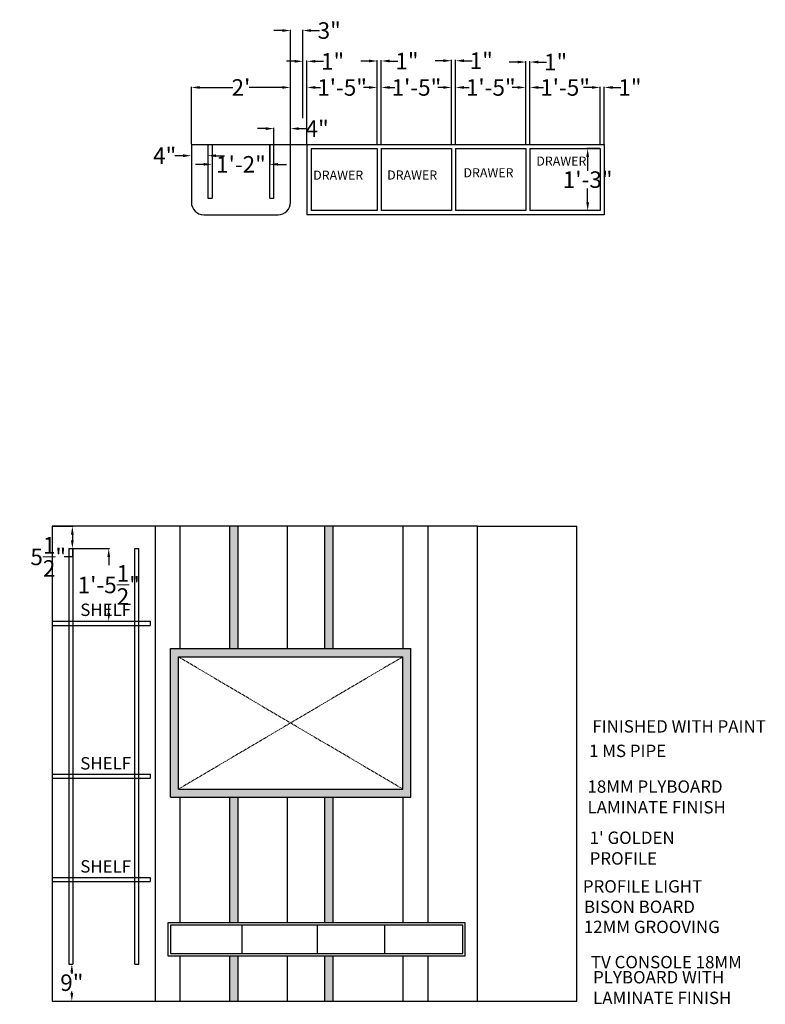
# Model space of a CAD drawing. Units: inches. Extents: x 40 to 220, y 34 to 272.
import ezdxf

# ---------------------------------------------------------------- set-up
doc = ezdxf.new("R2010")
doc.units = ezdxf.units.IN
doc.header["$MEASUREMENT"] = 0
doc.linetypes.add('CENTER2', pattern=[1.125, 0.75, -0.125, 0.125, -0.125])
for name, color, linetype, lineweight in [('A-ANNO-DIMS', 2, 'Continuous', 18), ('A-ANNO-TEXT', 7, 'Continuous', 18), ('A-EQPM', 8, 'CENTER2', 18), ('A-FURN', 7, 'Continuous', 25), ('A-FURN-PATT', 30, 'Continuous', 13)]:
    doc.layers.add(name, color=color, linetype=linetype, lineweight=lineweight)
doc.styles.get("Standard").update_dxf_attribs({"font": 'arial.ttf'})
doc.dimstyles.get("Standard").update_dxf_attribs({"dimtxt": 4, "dimasz": 2, "dimexe": 0.18, "dimexo": 0.0625, "dimgap": 0.09, "dimtad": 0, "dimtih": 1, "dimtoh": 1, "dimdec": 1, "dimzin": 0, "dimdsep": 46, "dimlunit": 4, "dimtxsty": 'Standard', "dimcen": 0.09, "dimadec": 0, "dimazin": 0, "dimtfac": 1, "dimtdec": 1, "dimtofl": 0, "dimtmove": 0, "dimatfit": 3, "dimfxl": 1, "dimtolj": 1, "dimtzin": 0, "dimarcsym": 1})

# ---------------------------------------------------------------- blocks, each defined once
blk = doc.blocks.new('*D1')
at = {"layer": 'A-ANNO-DIMS', "color": 0, "lineweight": -2, "transparency": 16777216}
for p, q in [((81.22, 241.93), (81.22, 255.87)), ((83.22, 255.69), (91.25, 255.69)), ((103.22, 255.69), (95.18, 255.69)), ((105.22, 241.93), (105.22, 255.87))]:
    blk.add_line(p, q, dxfattribs=at)
at = {"layer": 'A-ANNO-DIMS', "color": 0, "transparency": 16777216}
for points in [[(83.22, 256.02), (83.22, 255.36), (81.22, 255.69)], [(103.22, 256.02), (103.22, 255.36), (105.22, 255.69)]]:
    blk.add_solid(points, dxfattribs=at)
at = {"layer": 'Defpoints', "color": 0, "transparency": 16777216}
for p in [(105.22, 255.69), (81.22, 241.87), (105.22, 241.87)]:
    blk.add_point(p, dxfattribs=at)
at = {"layer": 'A-ANNO-DIMS', "color": 0, "transparency": 16777216, "insert": (93.22, 255.69), "char_height": 4, "attachment_point": 5}
blk.add_mtext("\\A1;2'", dxfattribs=at)
blk = doc.blocks.new('*D2')
at = {"layer": 'A-ANNO-DIMS', "color": 0, "lineweight": -2, "transparency": 16777216}
for p, q in [((103.22, 269.47), (101.22, 269.47)), ((105.22, 255.72), (105.22, 269.65)), ((108.22, 255.72), (108.22, 269.65)), ((110.22, 269.47), (112.22, 269.47))]:
    blk.add_line(p, q, dxfattribs=at)
at = {"layer": 'A-ANNO-DIMS', "color": 0, "transparency": 16777216}
for points in [[(103.22, 269.8), (103.22, 269.14), (105.22, 269.47)], [(110.22, 269.8), (110.22, 269.14), (108.22, 269.47)]]:
    blk.add_solid(points, dxfattribs=at)
at = {"layer": 'Defpoints', "color": 0, "transparency": 16777216}
for p in [(108.22, 269.47), (105.22, 255.65), (108.22, 255.65)]:
    blk.add_point(p, dxfattribs=at)
at = {"layer": 'A-ANNO-DIMS', "color": 0, "transparency": 16777216, "insert": (114.6, 269.47), "char_height": 4, "attachment_point": 5}
blk.add_mtext('\\A1;3"', dxfattribs=at)
blk = doc.blocks.new('*D3')
at = {"layer": 'A-ANNO-DIMS', "color": 0, "lineweight": -2, "transparency": 16777216}
for p, q in [((106.22, 262.02), (104.22, 262.02)), ((108.22, 248.27), (108.22, 262.2)), ((109.22, 248.27), (109.22, 262.2)), ((111.22, 262.02), (113.22, 262.02))]:
    blk.add_line(p, q, dxfattribs=at)
at = {"layer": 'A-ANNO-DIMS', "color": 0, "transparency": 16777216}
for points in [[(106.22, 262.35), (106.22, 261.69), (108.22, 262.02)], [(111.22, 262.35), (111.22, 261.69), (109.22, 262.02)]]:
    blk.add_solid(points, dxfattribs=at)
at = {"layer": 'Defpoints', "color": 0, "transparency": 16777216}
for p in [(109.22, 262.02), (108.22, 248.2), (109.22, 248.2)]:
    blk.add_point(p, dxfattribs=at)
at = {"layer": 'A-ANNO-DIMS', "color": 0, "transparency": 16777216, "insert": (115.42, 262.02), "char_height": 4, "attachment_point": 5}
blk.add_mtext('\\A1;1"', dxfattribs=at)
blk = doc.blocks.new('*D4')
at = {"layer": 'A-ANNO-DIMS', "color": 0, "lineweight": -2, "transparency": 16777216}
for p, q in [((109.22, 241.93), (109.22, 255.87)), ((111.22, 255.69), (112.5, 255.69)), ((124.22, 255.69), (122.93, 255.69)), ((126.22, 241.93), (126.22, 255.87))]:
    blk.add_line(p, q, dxfattribs=at)
at = {"layer": 'A-ANNO-DIMS', "color": 0, "transparency": 16777216}
for points in [[(111.22, 256.02), (111.22, 255.36), (109.22, 255.69)], [(124.22, 256.02), (124.22, 255.36), (126.22, 255.69)]]:
    blk.add_solid(points, dxfattribs=at)
at = {"layer": 'Defpoints', "color": 0, "transparency": 16777216}
for p in [(126.22, 255.69), (109.22, 241.87), (126.22, 241.87)]:
    blk.add_point(p, dxfattribs=at)
at = {"layer": 'A-ANNO-DIMS', "color": 0, "transparency": 16777216, "insert": (117.72, 255.69), "char_height": 4, "attachment_point": 5}
blk.add_mtext('\\A1;1\'-5"', dxfattribs=at)
blk = doc.blocks.new('*D5')
at = {"layer": 'A-ANNO-DIMS', "color": 0, "lineweight": -2, "transparency": 16777216}
for p, q in [((126.22, 248.34), (126.22, 262.27)), ((127.22, 248.34), (127.22, 262.27)), ((124.22, 262.09), (122.22, 262.09)), ((129.22, 262.09), (131.22, 262.09))]:
    blk.add_line(p, q, dxfattribs=at)
at = {"layer": 'A-ANNO-DIMS', "color": 0, "transparency": 16777216}
for points in [[(124.22, 262.43), (124.22, 261.76), (126.22, 262.09)], [(129.22, 262.43), (129.22, 261.76), (127.22, 262.09)]]:
    blk.add_solid(points, dxfattribs=at)
at = {"layer": 'Defpoints', "color": 0, "transparency": 16777216}
for p in [(127.22, 262.09), (126.22, 248.28), (127.22, 248.28)]:
    blk.add_point(p, dxfattribs=at)
at = {"layer": 'A-ANNO-DIMS', "color": 0, "transparency": 16777216, "insert": (133.42, 262.09), "char_height": 4, "attachment_point": 5}
blk.add_mtext('\\A1;1"', dxfattribs=at)
blk = doc.blocks.new('*D6')
at = {"layer": 'A-ANNO-DIMS', "color": 0, "lineweight": -2, "transparency": 16777216}
for p, q in [((127.22, 241.93), (127.22, 255.87)), ((129.22, 255.69), (130.5, 255.69)), ((142.22, 255.69), (140.93, 255.69)), ((144.22, 241.93), (144.22, 255.87))]:
    blk.add_line(p, q, dxfattribs=at)
at = {"layer": 'A-ANNO-DIMS', "color": 0, "transparency": 16777216}
for points in [[(129.22, 256.02), (129.22, 255.36), (127.22, 255.69)], [(142.22, 256.02), (142.22, 255.36), (144.22, 255.69)]]:
    blk.add_solid(points, dxfattribs=at)
at = {"layer": 'Defpoints', "color": 0, "transparency": 16777216}
for p in [(144.22, 255.69), (127.22, 241.87), (144.22, 241.87)]:
    blk.add_point(p, dxfattribs=at)
at = {"layer": 'A-ANNO-DIMS', "color": 0, "transparency": 16777216, "insert": (135.72, 255.69), "char_height": 4, "attachment_point": 5}
blk.add_mtext('\\A1;1\'-5"', dxfattribs=at)
blk = doc.blocks.new('*D7')
at = {"layer": 'A-ANNO-DIMS', "color": 0, "lineweight": -2, "transparency": 16777216}
for p, q in [((144.22, 248.41), (144.22, 262.34)), ((145.22, 248.41), (145.22, 262.34)), ((142.22, 262.16), (140.22, 262.16)), ((147.22, 262.16), (149.22, 262.16))]:
    blk.add_line(p, q, dxfattribs=at)
at = {"layer": 'A-ANNO-DIMS', "color": 0, "transparency": 16777216}
for points in [[(142.22, 262.5), (142.22, 261.83), (144.22, 262.16)], [(147.22, 262.5), (147.22, 261.83), (145.22, 262.16)]]:
    blk.add_solid(points, dxfattribs=at)
at = {"layer": 'Defpoints', "color": 0, "transparency": 16777216}
for p in [(145.22, 262.16), (144.22, 248.35), (145.22, 248.35)]:
    blk.add_point(p, dxfattribs=at)
at = {"layer": 'A-ANNO-DIMS', "color": 0, "transparency": 16777216, "insert": (151.42, 262.16), "char_height": 4, "attachment_point": 5}
blk.add_mtext('\\A1;1"', dxfattribs=at)
blk = doc.blocks.new('*D8')
at = {"layer": 'A-ANNO-DIMS', "color": 0, "lineweight": -2, "transparency": 16777216}
for p, q in [((145.22, 241.93), (145.22, 255.87)), ((147.22, 255.69), (148.5, 255.69)), ((160.22, 255.69), (158.93, 255.69)), ((162.22, 241.93), (162.22, 255.87))]:
    blk.add_line(p, q, dxfattribs=at)
at = {"layer": 'A-ANNO-DIMS', "color": 0, "transparency": 16777216}
for points in [[(147.22, 256.02), (147.22, 255.36), (145.22, 255.69)], [(160.22, 256.02), (160.22, 255.36), (162.22, 255.69)]]:
    blk.add_solid(points, dxfattribs=at)
at = {"layer": 'Defpoints', "color": 0, "transparency": 16777216}
for p in [(162.22, 255.69), (145.22, 241.87), (162.22, 241.87)]:
    blk.add_point(p, dxfattribs=at)
at = {"layer": 'A-ANNO-DIMS', "color": 0, "transparency": 16777216, "insert": (153.72, 255.69), "char_height": 4, "attachment_point": 5}
blk.add_mtext('\\A1;1\'-5"', dxfattribs=at)
blk = doc.blocks.new('*D9')
at = {"layer": 'A-ANNO-DIMS', "color": 0, "lineweight": -2, "transparency": 16777216}
for p, q in [((160.22, 261.84), (158.22, 261.84)), ((162.22, 248.08), (162.22, 262.02)), ((163.22, 248.08), (163.22, 262.02)), ((165.22, 261.84), (167.22, 261.84))]:
    blk.add_line(p, q, dxfattribs=at)
at = {"layer": 'A-ANNO-DIMS', "color": 0, "transparency": 16777216}
for points in [[(160.22, 262.17), (160.22, 261.51), (162.22, 261.84)], [(165.22, 262.17), (165.22, 261.51), (163.22, 261.84)]]:
    blk.add_solid(points, dxfattribs=at)
at = {"layer": 'Defpoints', "color": 0, "transparency": 16777216}
for p in [(163.22, 261.84), (162.22, 248.02), (163.22, 248.02)]:
    blk.add_point(p, dxfattribs=at)
at = {"layer": 'A-ANNO-DIMS', "color": 0, "transparency": 16777216, "insert": (169.42, 261.84), "char_height": 4, "attachment_point": 5}
blk.add_mtext('\\A1;1"', dxfattribs=at)
blk = doc.blocks.new('*D10')
at = {"layer": 'A-ANNO-DIMS', "color": 0, "lineweight": -2, "transparency": 16777216}
for p, q in [((163.22, 241.93), (163.22, 255.87)), ((165.22, 255.69), (166.5, 255.69)), ((178.22, 255.69), (176.93, 255.69)), ((180.22, 241.93), (180.22, 255.87))]:
    blk.add_line(p, q, dxfattribs=at)
at = {"layer": 'A-ANNO-DIMS', "color": 0, "transparency": 16777216}
for points in [[(165.22, 256.02), (165.22, 255.36), (163.22, 255.69)], [(178.22, 256.02), (178.22, 255.36), (180.22, 255.69)]]:
    blk.add_solid(points, dxfattribs=at)
at = {"layer": 'Defpoints', "color": 0, "transparency": 16777216}
for p in [(180.22, 255.69), (163.22, 241.87), (180.22, 241.87)]:
    blk.add_point(p, dxfattribs=at)
at = {"layer": 'A-ANNO-DIMS', "color": 0, "transparency": 16777216, "insert": (171.72, 255.69), "char_height": 4, "attachment_point": 5}
blk.add_mtext('\\A1;1\'-5"', dxfattribs=at)
blk = doc.blocks.new('*D11')
at = {"layer": 'A-ANNO-DIMS', "color": 0, "lineweight": -2, "transparency": 16777216}
for p, q in [((178.22, 255.69), (176.22, 255.69)), ((180.22, 241.93), (180.22, 255.87)), ((181.22, 241.93), (181.22, 255.87)), ((183.22, 255.69), (185.22, 255.69))]:
    blk.add_line(p, q, dxfattribs=at)
at = {"layer": 'A-ANNO-DIMS', "color": 0, "transparency": 16777216}
for points in [[(178.22, 256.02), (178.22, 255.36), (180.22, 255.69)], [(183.22, 256.02), (183.22, 255.36), (181.22, 255.69)]]:
    blk.add_solid(points, dxfattribs=at)
at = {"layer": 'Defpoints', "color": 0, "transparency": 16777216}
for p in [(181.22, 255.69), (180.22, 241.87), (181.22, 241.87)]:
    blk.add_point(p, dxfattribs=at)
at = {"layer": 'A-ANNO-DIMS', "color": 0, "transparency": 16777216, "insert": (187.42, 255.69), "char_height": 4, "attachment_point": 5}
blk.add_mtext('\\A1;1"', dxfattribs=at)
blk = doc.blocks.new('*D12')
at = {"layer": 'A-ANNO-DIMS', "color": 0, "lineweight": -2, "transparency": 16777216}
for p, q in [((99.22, 245.72), (97.22, 245.72)), ((101.22, 241.93), (101.22, 245.9)), ((105.22, 241.93), (105.22, 245.9)), ((107.22, 245.72), (109.22, 245.72))]:
    blk.add_line(p, q, dxfattribs=at)
at = {"layer": 'A-ANNO-DIMS', "color": 0, "transparency": 16777216}
for points in [[(99.22, 246.05), (99.22, 245.38), (101.22, 245.72)], [(107.22, 246.05), (107.22, 245.38), (105.22, 245.72)]]:
    blk.add_solid(points, dxfattribs=at)
at = {"layer": 'Defpoints', "color": 0, "transparency": 16777216}
for p in [(105.22, 245.72), (101.22, 241.87), (105.22, 241.87)]:
    blk.add_point(p, dxfattribs=at)
at = {"layer": 'A-ANNO-DIMS', "color": 0, "transparency": 16777216, "insert": (111.68, 245.72), "char_height": 4, "attachment_point": 5}
blk.add_mtext('\\A1;4"', dxfattribs=at)
blk = doc.blocks.new('*D13')
at = {"layer": 'A-ANNO-DIMS', "color": 0, "lineweight": -2, "transparency": 16777216}
for p, q in [((81.22, 241.81), (81.22, 238.98)), ((85.22, 241.81), (85.22, 238.98)), ((79.22, 239.16), (77.22, 239.16)), ((87.22, 239.16), (89.22, 239.16))]:
    blk.add_line(p, q, dxfattribs=at)
at = {"layer": 'A-ANNO-DIMS', "color": 0, "transparency": 16777216}
for points in [[(79.22, 239.5), (79.22, 238.83), (81.22, 239.16)], [(87.22, 239.5), (87.22, 238.83), (85.22, 239.16)]]:
    blk.add_solid(points, dxfattribs=at)
at = {"layer": 'Defpoints', "color": 0, "transparency": 16777216}
for p in [(81.22, 241.87), (85.22, 241.87), (81.22, 239.16)]:
    blk.add_point(p, dxfattribs=at)
at = {"layer": 'A-ANNO-DIMS', "color": 0, "transparency": 16777216, "insert": (74.75, 239.16), "char_height": 4, "attachment_point": 5}
blk.add_mtext('\\A1;4"', dxfattribs=at)
blk = doc.blocks.new('*D14')
at = {"layer": 'A-ANNO-DIMS', "color": 0, "lineweight": -2, "transparency": 16777216}
for p, q in [((86.22, 241.81), (86.22, 236.89)), ((100.22, 241.81), (100.22, 236.89)), ((84.22, 237.07), (82.22, 237.07)), ((102.22, 237.07), (104.22, 237.07))]:
    blk.add_line(p, q, dxfattribs=at)
at = {"layer": 'A-ANNO-DIMS', "color": 0, "transparency": 16777216}
for points in [[(84.22, 237.41), (84.22, 236.74), (86.22, 237.07)], [(102.22, 237.41), (102.22, 236.74), (100.22, 237.07)]]:
    blk.add_solid(points, dxfattribs=at)
at = {"layer": 'Defpoints', "color": 0, "transparency": 16777216}
for p in [(86.22, 241.87), (100.22, 241.87), (100.22, 237.07)]:
    blk.add_point(p, dxfattribs=at)
at = {"layer": 'A-ANNO-DIMS', "color": 0, "transparency": 16777216, "insert": (93.22, 237.07), "char_height": 4, "attachment_point": 5}
blk.add_mtext('\\A1;1\'-2"', dxfattribs=at)
blk = doc.blocks.new('*D15')
at = {"layer": 'A-ANNO-DIMS', "color": 0, "lineweight": -2, "transparency": 16777216}
for p, q in [((180.15, 240.87), (177.01, 240.87)), ((177.19, 238.87), (177.19, 235.51)), ((177.19, 227.87), (177.19, 231.24)), ((180.15, 225.87), (177.01, 225.87))]:
    blk.add_line(p, q, dxfattribs=at)
at = {"layer": 'A-ANNO-DIMS', "color": 0, "transparency": 16777216}
for points in [[(176.85, 238.87), (177.52, 238.87), (177.19, 240.87)], [(176.85, 227.87), (177.52, 227.87), (177.19, 225.87)]]:
    blk.add_solid(points, dxfattribs=at)
at = {"layer": 'Defpoints', "color": 0, "transparency": 16777216}
for p in [(180.22, 240.87), (177.19, 225.87), (180.22, 225.87)]:
    blk.add_point(p, dxfattribs=at)
at = {"layer": 'A-ANNO-DIMS', "color": 0, "transparency": 16777216, "insert": (177.19, 233.37), "char_height": 4, "attachment_point": 5}
blk.add_mtext('\\A1;1\'-3"', dxfattribs=at)
blk = doc.blocks.new('*D16')
at = {"layer": 'A-ANNO-DIMS', "color": 0, "lineweight": -2, "transparency": 16777216}
for p, q in [((47.59, 149.42), (52.58, 149.42)), ((52.4, 147.42), (52.4, 146.02)), ((51.59, 144.02), (52.58, 144.02)), ((52.4, 144.02), (52.4, 142.02)), ((52.4, 142.02), (50.4, 142.02))]:
    blk.add_line(p, q, dxfattribs=at)
at = {"layer": 'A-ANNO-DIMS', "color": 0, "transparency": 16777216}
for points in [[(52.06, 147.42), (52.73, 147.42), (52.4, 149.42)], [(52.06, 146.02), (52.73, 146.02), (52.4, 144.02)]]:
    blk.add_solid(points, dxfattribs=at)
at = {"layer": 'Defpoints', "color": 0, "transparency": 16777216}
for p in [(47.53, 149.42), (51.53, 144.02), (52.4, 144.02)]:
    blk.add_point(p, dxfattribs=at)
at = {"layer": 'A-ANNO-DIMS', "color": 0, "transparency": 16777216, "insert": (46.55, 142.02), "char_height": 4, "attachment_point": 5}
blk.add_mtext('\\A1;5{\\H1x;\\S1/2;}"', dxfattribs=at)
blk = doc.blocks.new('*D17')
at = {"layer": 'A-ANNO-DIMS', "color": 0, "lineweight": -2, "transparency": 16777216}
for p, q in [((52.64, 144.02), (61.39, 144.02)), ((61.21, 142.02), (61.21, 140.02)), ((61.21, 128.42), (61.21, 130.41)), ((52.64, 126.42), (61.39, 126.42))]:
    blk.add_line(p, q, dxfattribs=at)
at = {"layer": 'A-ANNO-DIMS', "color": 0, "transparency": 16777216}
for points in [[(60.88, 142.02), (61.54, 142.02), (61.21, 144.02)], [(60.88, 128.42), (61.54, 128.42), (61.21, 126.42)]]:
    blk.add_solid(points, dxfattribs=at)
at = {"layer": 'Defpoints', "color": 0, "transparency": 16777216}
for p in [(52.58, 144.02), (52.58, 126.42), (61.21, 126.42)]:
    blk.add_point(p, dxfattribs=at)
at = {"layer": 'A-ANNO-DIMS', "color": 0, "transparency": 16777216, "insert": (61.21, 135.22), "char_height": 4, "attachment_point": 5}
blk.add_mtext('\\A1;1\'-5{\\H1x;\\S1/2;}"', dxfattribs=at)
blk = doc.blocks.new('*D18')
at = {"layer": 'A-ANNO-DIMS', "color": 0, "lineweight": -2, "transparency": 16777216}
for p, q in [((51.59, 43.42), (52.45, 43.42)), ((52.27, 41.42), (52.27, 41.05)), ((52.27, 36.42), (52.27, 36.79)), ((47.59, 34.42), (52.45, 34.42))]:
    blk.add_line(p, q, dxfattribs=at)
at = {"layer": 'A-ANNO-DIMS', "color": 0, "transparency": 16777216}
for points in [[(51.94, 41.42), (52.61, 41.42), (52.27, 43.42)], [(51.94, 36.42), (52.61, 36.42), (52.27, 34.42)]]:
    blk.add_solid(points, dxfattribs=at)
at = {"layer": 'Defpoints', "color": 0, "transparency": 16777216}
for p in [(51.53, 43.42), (47.53, 34.42), (52.27, 34.42)]:
    blk.add_point(p, dxfattribs=at)
at = {"layer": 'A-ANNO-DIMS', "color": 0, "transparency": 16777216, "insert": (52.27, 38.92), "char_height": 4, "attachment_point": 5}
blk.add_mtext('\\A1;9"', dxfattribs=at)
blk = doc.blocks.new('DRAWER-FRONT')
for p, q in [((0, 15), (17, 15)), ((0, 15), (0, 0)), ((17, 15), (17, 0)), ((17, 0), (0, 0))]:
    blk.add_line(p, q)
blk = doc.blocks.new('SHELF')
for p, q in [((0, 1), (23.74, 1)), ((0, 0), (23.74, 0)), ((23.74, 1), (23.74, 0))]:
    blk.add_line(p, q)

msp = doc.modelspace()

# ---------------------------------------------------------------- hatches: boundary and pattern name
at = {"layer": 'A-FURN-PATT'}
h = msp.add_hatch(color=256, dxfattribs=at)
h.dxf.hatch_style = 1
h.paths.add_polyline_path([(92.53, 149.42), (90.53, 149.42), (90.53, 119.81), (92.53, 119.81)])
h.paths.add_polyline_path([(115.53, 149.42), (113.53, 149.42), (113.53, 119.81), (115.53, 119.81)])
h.paths.add_polyline_path([(92.53, 83.81), (90.53, 83.81), (90.53, 53.42), (92.53, 53.42)])
h.paths.add_polyline_path([(115.53, 83.81), (113.53, 83.81), (113.53, 53.42), (115.53, 53.42)])
h.paths.add_polyline_path([(115.53, 45.42), (113.53, 45.42), (113.53, 34.42), (115.53, 34.42)])
h.paths.add_polyline_path([(92.53, 45.42), (90.53, 45.42), (90.53, 34.42), (92.53, 34.42)])
h = msp.add_hatch(color=256, dxfattribs=at)
h.dxf.hatch_style = 1
h.paths.add_polyline_path([(134.39, 119.81), (76.13, 119.81), (76.13, 83.81), (134.39, 83.81)])
h.paths.add_polyline_path([(132.39, 117.81), (132.39, 85.81), (78.13, 85.81), (78.13, 117.81)], flags=16)

# ---------------------------------------------------------------- linework, layer by layer
at = {"layer": 'A-EQPM'}
for p, q in [((78.13, 117.81), (132.39, 85.81)), ((132.39, 117.81), (78.13, 85.81))]:
    msp.add_line(p, q, dxfattribs=at)
at = {"layer": 'A-FURN'}
for p, q in [((81.22, 241.87), (105.22, 241.87)), ((81.22, 241.87), (81.22, 227.87)), ((85.22, 241.87), (85.22, 228.87)), ((86.22, 241.87), (86.22, 228.87)), ((100.22, 228.87), (100.22, 241.87)), ((101.22, 228.87), (101.22, 241.87)), ((105.22, 241.87), (108.22, 241.87)), ((105.22, 227.87), (105.22, 241.87)), ((108.22, 241.87), (109.22, 241.87)), ((109.22, 241.87), (126.22, 241.87)), ((109.22, 241.87), (109.22, 224.87)), ((110.22, 240.87), (110.22, 225.87)), ((110.22, 240.87), (126.22, 240.87)), ((126.22, 241.87), (127.22, 241.87)), ((126.22, 240.87), (126.22, 225.87)), ((127.22, 241.87), (144.22, 241.87)), ((144.22, 241.87), (145.22, 241.87)), ((145.22, 241.87), (162.22, 241.87)), ((162.22, 241.87), (163.22, 241.87)), ((163.22, 241.87), (180.22, 241.87)), ((180.22, 241.87), (181.22, 241.87)), ((181.22, 241.87), (181.22, 224.87)), ((85.22, 228.87), (86.22, 228.87)), ((100.22, 228.87), (101.22, 228.87)), ((84.22, 224.87), (102.22, 224.87)), ((181.22, 224.87), (109.22, 224.87)), ((126.22, 225.87), (110.22, 225.87)), ((72.53, 149.42), (47.53, 149.42)), ((47.53, 149.42), (47.53, 34.42)), ((72.53, 34.42), (72.53, 149.42)), ((150.53, 149.42), (72.53, 149.42)), ((78.53, 119.81), (78.53, 149.42)), ((90.53, 119.81), (90.53, 149.42)), ((92.53, 119.81), (92.53, 149.42)), ((104.53, 119.81), (104.53, 149.42)), ((113.53, 119.81), (113.53, 149.42)), ((115.53, 119.81), (115.53, 149.42)), ((132.53, 119.81), (132.53, 149.42)), ((138.53, 53.42), (138.53, 149.42)), ((150.53, 34.42), (150.53, 149.42)), ((150.53, 149.42), (174.53, 149.42)), ((174.53, 34.42), (174.53, 149.42)), ((51.53, 144.02), (52.53, 144.02)), ((51.53, 144.02), (51.53, 43.42)), ((52.53, 144.02), (52.53, 43.42)), ((67.53, 43.42), (67.53, 144.02)), ((67.53, 144.02), (68.53, 144.02)), ((68.53, 43.42), (68.53, 144.02)), ((76.13, 83.81), (76.13, 119.81)), ((76.13, 119.81), (134.39, 119.81)), ((134.39, 83.81), (134.39, 119.81)), ((78.13, 117.81), (132.39, 117.81)), ((78.13, 85.81), (78.13, 117.81)), ((132.39, 85.81), (132.39, 117.81)), ((76.13, 83.81), (134.39, 83.81)), ((78.13, 85.81), (132.39, 85.81)), ((78.53, 53.42), (78.53, 83.81)), ((90.53, 53.42), (90.53, 83.81)), ((92.53, 53.42), (92.53, 83.81)), ((104.53, 53.42), (104.53, 83.81)), ((113.53, 53.42), (113.53, 83.81)), ((115.53, 53.42), (115.53, 83.81)), ((132.53, 53.42), (132.53, 83.81)), ((138.53, 53.42), (138.53, 83.81)), ((93.45, 52.82), (93.45, 46.02)), ((111.7, 52.82), (111.7, 46.02)), ((127.99, 52.82), (127.99, 46.02)), ((78.53, 34.42), (78.53, 45.42)), ((90.53, 34.42), (90.53, 45.42)), ((92.53, 34.42), (92.53, 45.42)), ((104.53, 34.42), (104.53, 45.42)), ((113.53, 34.42), (113.53, 45.42)), ((115.53, 34.42), (115.53, 45.42)), ((132.53, 34.42), (132.53, 45.42)), ((138.53, 34.42), (138.53, 45.42)), ((51.53, 43.42), (52.53, 43.42)), ((67.53, 43.42), (68.53, 43.42)), ((47.53, 34.42), (72.53, 34.42)), ((72.53, 34.42), (78.53, 34.42)), ((78.53, 34.42), (90.53, 34.42)), ((90.53, 34.42), (92.53, 34.42)), ((92.53, 34.42), (104.53, 34.42)), ((104.53, 34.42), (113.53, 34.42)), ((113.53, 34.42), (115.53, 34.42)), ((115.53, 34.42), (132.53, 34.42)), ((132.53, 34.42), (138.53, 34.42)), ((138.53, 34.42), (150.53, 34.42)), ((150.53, 34.42), (174.53, 34.42))]:
    msp.add_line(p, q, dxfattribs=at)
for points in [[(104.53, 53.42), (90.53, 53.42), (78.53, 53.42), (75.53, 53.42), (75.53, 45.42), (78.53, 45.42), (90.53, 45.42), (104.53, 45.42), (115.53, 45.42), (132.53, 45.42), (138.53, 45.42), (147.53, 45.42), (147.53, 53.42), (138.53, 53.42), (132.53, 53.42), (115.53, 53.42), (92.53, 53.42)], [(92.53, 52.82), (90.53, 52.82), (78.53, 52.82), (76.13, 52.82), (76.13, 46.02), (78.53, 46.02), (90.53, 46.02), (104.53, 46.02), (115.53, 46.02), (132.53, 46.02), (138.53, 46.02), (146.93, 46.02), (146.93, 52.82), (138.53, 52.82), (132.53, 52.82), (115.53, 52.82), (76.13, 52.82)]]:
    msp.add_lwpolyline(points, dxfattribs=at)
for centre, start, end in [((84.22, 227.87), 180, 270), ((102.22, 227.87), 270, 0)]:
    msp.add_arc(centre, 3, start, end, dxfattribs=at)

# ---------------------------------------------------------------- block references
for name, p in [('DRAWER-FRONT', (127.22, 225.87)), ('DRAWER-FRONT', (145.22, 225.87)), ('DRAWER-FRONT', (163.22, 225.87)), ('SHELF', (47.53, 125.42)), ('SHELF', (47.53, 88.42)), ('SHELF', (47.53, 63.42))]:
    msp.add_blockref(name, p, dxfattribs=at)

# ---------------------------------------------------------------- texts
at = {"layer": 'A-ANNO-TEXT', "attachment_point": 1}
for s, width, gutter_width, insert, char_height in [('DRAWER', 11.5035, 11, (164.77, 238.96), 2.2), ('DRAWER', 11.5035, 11, (147.12, 236.14), 2.2), ('DRAWER', 11.5035, 11, (110.73, 235.55), 2.2), ('DRAWER', 11.5035, 11, (128.64, 235.59), 2.2), ('SHELF', 12.4336, 15, (54.31, 130.71), 3), ('FINISHED WITH PAINT', 56.6049, 15, (178.33, 102.48), 3), ('1 MS PIPE', 59.8585, 15, (177.53, 96.55), 3), ('SHELF', 12.4336, 15, (54.31, 93.54), 3), ('18MM PLYBOARD\\PLAMINATE FINISH', 49.19, 15, (177.15, 87.9), 3), ("1' GOLDEN \\PPROFILE", 44.5195, 15, (177.67, 75.51), 3), ('SHELF', 12.4336, 15, (54.31, 68.58), 3), ('PROFILE LIGHT', 47.5036, 15, (176.02, 63.74), 3), ('BISON BOARD', 34.9324, 15, (176.3, 58.79), 3), ('12MM GROOVING', 39.0031, 15, (176.26, 53.93), 3), ('TV CONSOLE 18MM', 48.7855, 15, (177.99, 45.4), 3), ('PLYBOARD WITH \\PLAMINATE FINISH', 56.8195, 15, (178.5, 41.74), 3)]:
    msp.add_mtext_dynamic_manual_height_columns(s, width=width, gutter_width=gutter_width, heights=[0], dxfattribs=dict(at, insert=insert, char_height=char_height))

# ---------------------------------------------------------------- dimensions: what is measured, and where the dimension line sits
at = {"layer": 'A-ANNO-DIMS'}
for base, p1, p2, picture, middle in [((108.22, 269.47), (105.22, 255.65), (108.22, 255.65), '*D2', (114.6, 269.47)), ((109.22, 262.02), (108.22, 248.2), (109.22, 248.2), '*D3', (115.42, 262.02)), ((127.22, 262.09), (126.22, 248.28), (127.22, 248.28), '*D5', (133.42, 262.09)), ((145.22, 262.16), (144.22, 248.35), (145.22, 248.35), '*D7', (151.42, 262.16)), ((163.22, 261.84), (162.22, 248.02), (163.22, 248.02), '*D9', (169.42, 261.84)), ((105.22, 255.69), (81.22, 241.87), (105.22, 241.87), '*D1', (93.22, 255.69)), ((126.22, 255.69), (109.22, 241.87), (126.22, 241.87), '*D4', (117.72, 255.69)), ((144.22, 255.69), (127.22, 241.87), (144.22, 241.87), '*D6', (135.72, 255.69)), ((162.22, 255.69), (145.22, 241.87), (162.22, 241.87), '*D8', (153.72, 255.69)), ((180.22, 255.69), (163.22, 241.87), (180.22, 241.87), '*D10', (171.72, 255.69)), ((181.22, 255.69), (180.22, 241.87), (181.22, 241.87), '*D11', (187.42, 255.69)), ((105.22, 245.72), (101.22, 241.87), (105.22, 241.87), '*D12', (111.68, 245.72)), ((81.22, 239.16), (85.22, 241.87), (81.22, 241.87), '*D13', (74.75, 239.16)), ((100.22, 237.07), (86.22, 241.87), (100.22, 241.87), '*D14', (93.22, 237.07))]:
    dim = msp.add_linear_dim(base=base, p1=p1, p2=p2, dimstyle='Standard', override={"dimclrd": 0, "dimclre": 0, "dimclrt": 0}, dxfattribs=at)
    dim.commit()
    dim.dimension.update_dxf_attribs({"geometry": picture, "text_midpoint": middle})
for base, p1, p2, picture, middle in [((177.19, 225.87), (180.22, 240.87), (180.22, 225.87), '*D15', (177.19, 233.37)), ((52.4, 144.02), (47.53, 149.42), (51.53, 144.02), '*D16', (46.55, 142.02)), ((61.21, 126.42), (52.58, 144.02), (52.58, 126.42), '*D17', (61.21, 135.22)), ((52.27, 34.42), (51.53, 43.42), (47.53, 34.42), '*D18', (52.27, 38.92))]:
    dim = msp.add_linear_dim(base=base, p1=p1, p2=p2, angle=90, dimstyle='Standard', override={"dimclrd": 0, "dimclre": 0, "dimclrt": 0}, dxfattribs=at)
    dim.commit()
    dim.dimension.update_dxf_attribs({"geometry": picture, "text_midpoint": middle})

doc.saveas('drawing.dxf')
